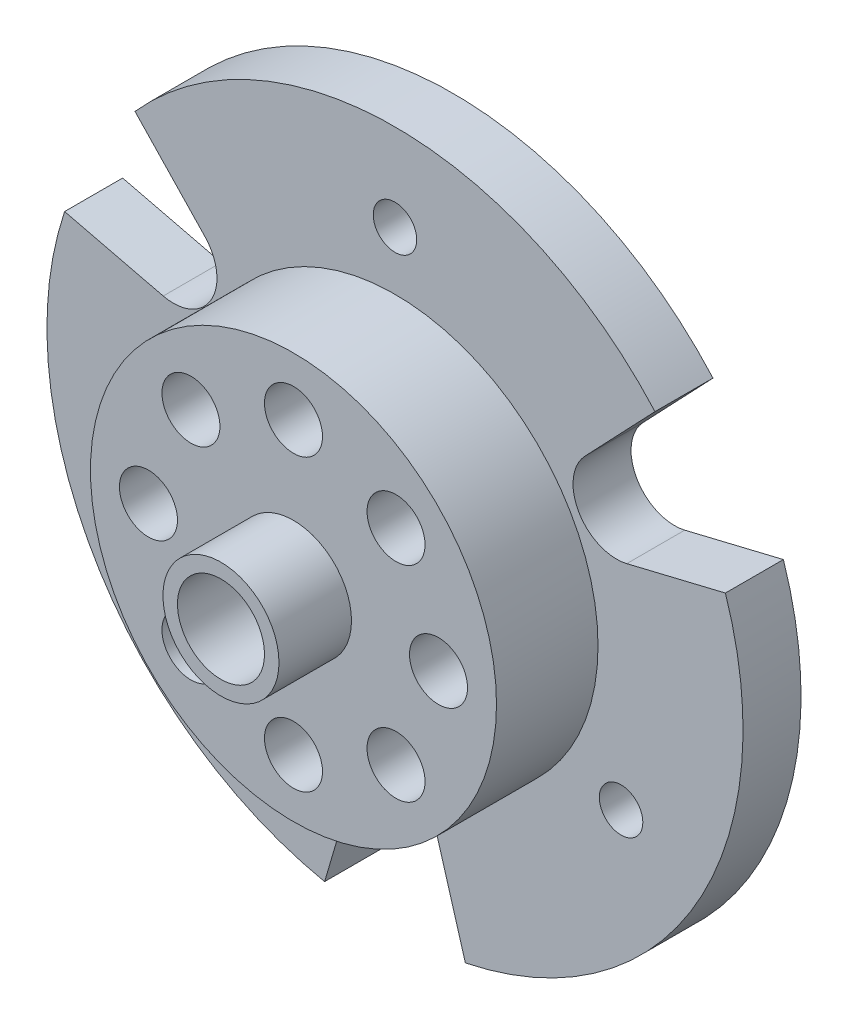
ISO-10303-21;
HEADER;
FILE_DESCRIPTION(('STEP AP214'),'2;1');
FILE_NAME('part.step','',(''),(''),'','','');
FILE_SCHEMA(('AUTOMOTIVE_DESIGN { 1 0 10303 214 1 1 1 1 }'));
ENDSEC;
DATA;
#1=APPLICATION_CONTEXT('core data for automotive mechanical design processes');
#2=APPLICATION_PROTOCOL_DEFINITION('international standard','automotive_design',2000,#1);
#3=PRODUCT_CONTEXT('',#1,'mechanical');
#4=PRODUCT('Part','Part','',(#3));
#5=PRODUCT_RELATED_PRODUCT_CATEGORY('part','',(#4));
#6=PRODUCT_DEFINITION_FORMATION('','',#4);
#7=PRODUCT_DEFINITION_CONTEXT('part definition',#1,'design');
#8=PRODUCT_DEFINITION('design','',#6,#7);
#9=PRODUCT_DEFINITION_SHAPE('','',#8);
#10=(LENGTH_UNIT() NAMED_UNIT(*) SI_UNIT(.MILLI.,.METRE.));
#11=(NAMED_UNIT(*) PLANE_ANGLE_UNIT() SI_UNIT($,.RADIAN.));
#12=(NAMED_UNIT(*) SI_UNIT($,.STERADIAN.) SOLID_ANGLE_UNIT());
#13=UNCERTAINTY_MEASURE_WITH_UNIT(LENGTH_MEASURE(1.E-05),#10,'distance_accuracy_value','');
#14=(GEOMETRIC_REPRESENTATION_CONTEXT(3) GLOBAL_UNCERTAINTY_ASSIGNED_CONTEXT((#13)) GLOBAL_UNIT_ASSIGNED_CONTEXT((#10,
#11,#12)) REPRESENTATION_CONTEXT('',''));
#15=CARTESIAN_POINT('',(0.,0.,0.));
#16=DIRECTION('',(0.,0.,1.));
#17=DIRECTION('',(1.,0.,0.));
#18=AXIS2_PLACEMENT_3D('',#15,#16,#17);
#19=CARTESIAN_POINT('',(0.,0.,4.));
#20=DIRECTION('',(0.,0.,-1.));
#21=DIRECTION('',(-1.,0.,0.));
#22=AXIS2_PLACEMENT_3D('',#19,#20,#21);
#23=CYLINDRICAL_SURFACE('',#22,24.);
#24=DIRECTION('',(0.,0.,1.));
#25=VECTOR('',#24,1.);
#26=CARTESIAN_POINT('',(-17.9280987104658,15.9556659725564,-26.));
#27=LINE('',#26,#25);
#28=CARTESIAN_POINT('',(-17.9280987104658,15.9556659725564,0.));
#29=VERTEX_POINT('',#28);
#30=CARTESIAN_POINT('',(-17.9280987104658,15.9556659725564,4.));
#31=VERTEX_POINT('',#30);
#32=EDGE_CURVE('E172',#29,#31,#27,.T.);
#33=ORIENTED_EDGE('',*,*,#32,.T.);
#34=CARTESIAN_POINT('',(0.,0.,4.));
#35=DIRECTION('',(0.,0.,1.));
#36=DIRECTION('',(1.,0.,0.));
#37=AXIS2_PLACEMENT_3D('',#34,#35,#36);
#38=CIRCLE('',#37,24.);
#39=CARTESIAN_POINT('',(17.928098710466,15.9556659725562,4.));
#40=VERTEX_POINT('',#39);
#41=EDGE_CURVE('E286',#40,#31,#38,.T.);
#42=ORIENTED_EDGE('',*,*,#41,.F.);
#43=DIRECTION('',(0.,0.,1.));
#44=VECTOR('',#43,1.);
#45=CARTESIAN_POINT('',(17.928098710466,15.9556659725562,-26.));
#46=LINE('',#45,#44);
#47=CARTESIAN_POINT('',(17.928098710466,15.9556659725562,0.));
#48=VERTEX_POINT('',#47);
#49=EDGE_CURVE('E162',#48,#40,#46,.T.);
#50=ORIENTED_EDGE('',*,*,#49,.F.);
#51=CARTESIAN_POINT('',(0.,0.,0.));
#52=DIRECTION('',(0.,0.,1.));
#53=DIRECTION('',(1.,0.,0.));
#54=AXIS2_PLACEMENT_3D('',#51,#52,#53);
#55=CIRCLE('',#54,24.);
#56=EDGE_CURVE('E291',#48,#29,#55,.T.);
#57=ORIENTED_EDGE('',*,*,#56,.T.);
#58=EDGE_LOOP('',(#33,#42,#50,#57));
#59=FACE_BOUND('',#58,.T.);
#60=ADVANCED_FACE('F60',(#59),#23,.T.);
#61=DIRECTION('',(0.,0.,1.));
#62=VECTOR('',#61,1.);
#63=CARTESIAN_POINT('',(22.7820614217657,7.5483559385401,-26.));
#64=LINE('',#63,#62);
#65=CARTESIAN_POINT('',(22.7820614217657,7.5483559385401,0.));
#66=VERTEX_POINT('',#65);
#67=CARTESIAN_POINT('',(22.7820614217657,7.5483559385401,4.));
#68=VERTEX_POINT('',#67);
#69=EDGE_CURVE('E187',#66,#68,#64,.T.);
#70=ORIENTED_EDGE('',*,*,#69,.T.);
#71=CARTESIAN_POINT('',(4.85396271129979,-23.5040219110966,4.));
#72=VERTEX_POINT('',#71);
#73=EDGE_CURVE('E289',#72,#68,#38,.T.);
#74=ORIENTED_EDGE('',*,*,#73,.F.);
#75=DIRECTION('',(0.,0.,1.));
#76=VECTOR('',#75,1.);
#77=CARTESIAN_POINT('',(4.85396271129979,-23.5040219110966,-26.));
#78=LINE('',#77,#76);
#79=CARTESIAN_POINT('',(4.85396271129979,-23.5040219110966,0.));
#80=VERTEX_POINT('',#79);
#81=EDGE_CURVE('E182',#80,#72,#78,.T.);
#82=ORIENTED_EDGE('',*,*,#81,.F.);
#83=EDGE_CURVE('E284',#80,#66,#55,.T.);
#84=ORIENTED_EDGE('',*,*,#83,.T.);
#85=EDGE_LOOP('',(#70,#74,#82,#84));
#86=FACE_BOUND('',#85,.T.);
#87=ADVANCED_FACE('F347',(#86),#23,.T.);
#88=CARTESIAN_POINT('',(-22.7820614217656,7.54835593854042,4.));
#89=VERTEX_POINT('',#88);
#90=CARTESIAN_POINT('',(-4.85396271129979,-23.5040219110967,4.));
#91=VERTEX_POINT('',#90);
#92=EDGE_CURVE('E295',#89,#91,#38,.T.);
#93=ORIENTED_EDGE('',*,*,#92,.F.);
#94=DIRECTION('',(0.,0.,1.));
#95=VECTOR('',#94,1.);
#96=CARTESIAN_POINT('',(-22.7820614217656,7.54835593854042,-26.));
#97=LINE('',#96,#95);
#98=CARTESIAN_POINT('',(-22.7820614217656,7.54835593854042,0.));
#99=VERTEX_POINT('',#98);
#100=EDGE_CURVE('E157',#99,#89,#97,.T.);
#101=ORIENTED_EDGE('',*,*,#100,.F.);
#102=CARTESIAN_POINT('',(-4.85396271129979,-23.5040219110967,0.));
#103=VERTEX_POINT('',#102);
#104=EDGE_CURVE('E298',#99,#103,#55,.T.);
#105=ORIENTED_EDGE('',*,*,#104,.T.);
#106=DIRECTION('',(0.,0.,1.));
#107=VECTOR('',#106,1.);
#108=CARTESIAN_POINT('',(-4.85396271129979,-23.5040219110967,-26.));
#109=LINE('',#108,#107);
#110=EDGE_CURVE('E204',#103,#91,#109,.T.);
#111=ORIENTED_EDGE('',*,*,#110,.T.);
#112=EDGE_LOOP('',(#93,#101,#105,#111));
#113=FACE_BOUND('',#112,.T.);
#114=ADVANCED_FACE('F56',(#113),#23,.T.);
#115=CARTESIAN_POINT('',(0.,0.,4.));
#116=DIRECTION('',(0.,0.,1.));
#117=DIRECTION('',(1.,0.,0.));
#118=AXIS2_PLACEMENT_3D('',#115,#116,#117);
#119=PLANE('',#118);
#120=DIRECTION('',(0.97198847965738,-0.235028499151349,0.));
#121=VECTOR('',#120,1.);
#122=CARTESIAN_POINT('',(0.465939606669434,1.92694899356498,4.));
#123=LINE('',#122,#121);
#124=CARTESIAN_POINT('',(-15.9817736202115,5.90403456102793,4.));
#125=VERTEX_POINT('',#124);
#126=EDGE_CURVE('E156',#89,#125,#123,.T.);
#127=ORIENTED_EDGE('',*,*,#126,.F.);
#128=ORIENTED_EDGE('',*,*,#92,.T.);
#129=DIRECTION('',(0.282453588950297,0.959280965144778,0.));
#130=VECTOR('',#129,1.);
#131=CARTESIAN_POINT('',(1.90175658355885,-0.559958960777444,4.));
#132=LINE('',#131,#130);
#133=CARTESIAN_POINT('',(-2.87784289543433,-16.7926392331491,4.));
#134=VERTEX_POINT('',#133);
#135=EDGE_CURVE('E200',#91,#134,#132,.T.);
#136=ORIENTED_EDGE('',*,*,#135,.T.);
#137=CARTESIAN_POINT('',(0.,-17.64,4.));
#138=DIRECTION('',(0.,0.,1.));
#139=DIRECTION('',(1.,0.,0.));
#140=AXIS2_PLACEMENT_3D('',#137,#138,#139);
#141=CIRCLE('',#140,3.);
#142=CARTESIAN_POINT('',(2.87784289543436,-16.7926392331492,4.));
#143=VERTEX_POINT('',#142);
#144=EDGE_CURVE('E198',#143,#134,#141,.T.);
#145=ORIENTED_EDGE('',*,*,#144,.F.);
#146=DIRECTION('',(-0.282453588950297,0.959280965144778,0.));
#147=VECTOR('',#146,1.);
#148=CARTESIAN_POINT('',(-1.90175658355885,-0.559958960777445,4.));
#149=LINE('',#148,#147);
#150=EDGE_CURVE('E191',#72,#143,#149,.T.);
#151=ORIENTED_EDGE('',*,*,#150,.F.);
#152=ORIENTED_EDGE('',*,*,#73,.T.);
#153=DIRECTION('',(-0.971988479657383,-0.235028499151335,0.));
#154=VECTOR('',#153,1.);
#155=CARTESIAN_POINT('',(-0.465939606669407,1.92694899356499,4.));
#156=LINE('',#155,#154);
#157=CARTESIAN_POINT('',(15.9817736202116,5.90403456102771,4.));
#158=VERTEX_POINT('',#157);
#159=EDGE_CURVE('E181',#68,#158,#156,.T.);
#160=ORIENTED_EDGE('',*,*,#159,.T.);
#161=CARTESIAN_POINT('',(15.2766881227576,8.81999999999986,4.));
#162=DIRECTION('',(0.,0.,1.));
#163=DIRECTION('',(1.,0.,0.));
#164=AXIS2_PLACEMENT_3D('',#161,#162,#163);
#165=CIRCLE('',#164,3.);
#166=CARTESIAN_POINT('',(13.1039307247773,10.8886046721211,4.));
#167=VERTEX_POINT('',#166);
#168=EDGE_CURVE('E177',#167,#158,#165,.T.);
#169=ORIENTED_EDGE('',*,*,#168,.F.);
#170=DIRECTION('',(-0.689534890707091,-0.724252465993427,0.));
#171=VECTOR('',#170,1.);
#172=CARTESIAN_POINT('',(1.43581697688941,-1.36699003278756,4.));
#173=LINE('',#172,#171);
#174=EDGE_CURVE('E180',#40,#167,#173,.T.);
#175=ORIENTED_EDGE('',*,*,#174,.F.);
#176=ORIENTED_EDGE('',*,*,#41,.T.);
#177=DIRECTION('',(0.689534890707081,-0.724252465993437,0.));
#178=VECTOR('',#177,1.);
#179=CARTESIAN_POINT('',(-1.43581697688943,-1.36699003278754,4.));
#180=LINE('',#179,#178);
#181=CARTESIAN_POINT('',(-13.1039307247772,10.8886046721213,4.));
#182=VERTEX_POINT('',#181);
#183=EDGE_CURVE('E153',#31,#182,#180,.T.);
#184=ORIENTED_EDGE('',*,*,#183,.T.);
#185=CARTESIAN_POINT('',(-15.2766881227575,8.82,4.));
#186=DIRECTION('',(0.,0.,1.));
#187=DIRECTION('',(1.,0.,0.));
#188=AXIS2_PLACEMENT_3D('',#185,#186,#187);
#189=CIRCLE('',#188,3.);
#190=EDGE_CURVE('E146',#125,#182,#189,.T.);
#191=ORIENTED_EDGE('',*,*,#190,.F.);
#192=EDGE_LOOP('',(#127,#128,#136,#145,#151,#152,#160,#169,#175,#176,#184,#191));
#193=FACE_BOUND('',#192,.T.);
#194=CARTESIAN_POINT('',(-15.5884572681187,-9.00000000000067,4.));
#195=DIRECTION('',(0.,0.,1.));
#196=DIRECTION('',(1.,0.,0.));
#197=AXIS2_PLACEMENT_3D('',#194,#195,#196);
#198=CIRCLE('',#197,1.50000000000146);
#199=CARTESIAN_POINT('',(-14.0884572681173,-9.00000000000067,4.));
#200=VERTEX_POINT('',#199);
#201=EDGE_CURVE('E269',#200,#200,#198,.T.);
#202=ORIENTED_EDGE('',*,*,#201,.F.);
#203=EDGE_LOOP('',(#202));
#204=FACE_BOUND('',#203,.T.);
#205=CARTESIAN_POINT('',(15.588457268121,-8.99999999999934,4.));
#206=DIRECTION('',(0.,0.,1.));
#207=DIRECTION('',(1.,0.,0.));
#208=AXIS2_PLACEMENT_3D('',#205,#206,#207);
#209=CIRCLE('',#208,1.50000000000099);
#210=CARTESIAN_POINT('',(17.088457268122,-8.99999999999934,4.));
#211=VERTEX_POINT('',#210);
#212=EDGE_CURVE('E273',#211,#211,#209,.T.);
#213=ORIENTED_EDGE('',*,*,#212,.F.);
#214=EDGE_LOOP('',(#213));
#215=FACE_BOUND('',#214,.T.);
#216=CARTESIAN_POINT('',(0.,18.,4.));
#217=DIRECTION('',(0.,0.,1.));
#218=DIRECTION('',(1.,0.,0.));
#219=AXIS2_PLACEMENT_3D('',#216,#217,#218);
#220=CIRCLE('',#219,1.5);
#221=CARTESIAN_POINT('',(1.5,18.,4.));
#222=VERTEX_POINT('',#221);
#223=EDGE_CURVE('E270',#222,#222,#220,.T.);
#224=ORIENTED_EDGE('',*,*,#223,.F.);
#225=EDGE_LOOP('',(#224));
#226=FACE_BOUND('',#225,.T.);
#227=CARTESIAN_POINT('',(0.,0.,4.));
#228=DIRECTION('',(0.,0.,1.));
#229=DIRECTION('',(1.,0.,0.));
#230=AXIS2_PLACEMENT_3D('',#227,#228,#229);
#231=CIRCLE('',#230,14.);
#232=CARTESIAN_POINT('',(14.,0.,4.));
#233=VERTEX_POINT('',#232);
#234=EDGE_CURVE('E285',#233,#233,#231,.T.);
#235=ORIENTED_EDGE('',*,*,#234,.F.);
#236=EDGE_LOOP('',(#235));
#237=FACE_BOUND('',#236,.T.);
#238=ADVANCED_FACE('F164',(#193,#204,#215,#226,#237),#119,.T.);
#239=CARTESIAN_POINT('',(0.,0.,0.));
#240=DIRECTION('',(0.,0.,1.));
#241=DIRECTION('',(1.,0.,0.));
#242=AXIS2_PLACEMENT_3D('',#239,#240,#241);
#243=PLANE('',#242);
#244=CARTESIAN_POINT('',(0.,0.,0.));
#245=DIRECTION('',(0.,0.,1.));
#246=DIRECTION('',(1.,0.,0.));
#247=AXIS2_PLACEMENT_3D('',#244,#245,#246);
#248=CIRCLE('',#247,3.);
#249=CARTESIAN_POINT('',(3.,0.,0.));
#250=VERTEX_POINT('',#249);
#251=EDGE_CURVE('E215',#250,#250,#248,.T.);
#252=ORIENTED_EDGE('',*,*,#251,.T.);
#253=EDGE_LOOP('',(#252));
#254=FACE_BOUND('',#253,.T.);
#255=CARTESIAN_POINT('',(-15.5884572681187,-9.00000000000067,0.));
#256=DIRECTION('',(0.,0.,1.));
#257=DIRECTION('',(1.,0.,0.));
#258=AXIS2_PLACEMENT_3D('',#255,#256,#257);
#259=CIRCLE('',#258,1.50000000000146);
#260=CARTESIAN_POINT('',(-14.0884572681173,-9.00000000000067,0.));
#261=VERTEX_POINT('',#260);
#262=EDGE_CURVE('E282',#261,#261,#259,.T.);
#263=ORIENTED_EDGE('',*,*,#262,.T.);
#264=EDGE_LOOP('',(#263));
#265=FACE_BOUND('',#264,.T.);
#266=CARTESIAN_POINT('',(15.588457268121,-8.99999999999934,0.));
#267=DIRECTION('',(0.,0.,1.));
#268=DIRECTION('',(1.,0.,0.));
#269=AXIS2_PLACEMENT_3D('',#266,#267,#268);
#270=CIRCLE('',#269,1.50000000000099);
#271=CARTESIAN_POINT('',(17.088457268122,-8.99999999999934,0.));
#272=VERTEX_POINT('',#271);
#273=EDGE_CURVE('E300',#272,#272,#270,.T.);
#274=ORIENTED_EDGE('',*,*,#273,.T.);
#275=EDGE_LOOP('',(#274));
#276=FACE_BOUND('',#275,.T.);
#277=CARTESIAN_POINT('',(0.,18.,0.));
#278=DIRECTION('',(0.,0.,1.));
#279=DIRECTION('',(1.,0.,0.));
#280=AXIS2_PLACEMENT_3D('',#277,#278,#279);
#281=CIRCLE('',#280,1.5);
#282=CARTESIAN_POINT('',(1.5,18.,0.));
#283=VERTEX_POINT('',#282);
#284=EDGE_CURVE('E272',#283,#283,#281,.T.);
#285=ORIENTED_EDGE('',*,*,#284,.T.);
#286=EDGE_LOOP('',(#285));
#287=FACE_BOUND('',#286,.T.);
#288=ORIENTED_EDGE('',*,*,#104,.F.);
#289=DIRECTION('',(0.97198847965738,-0.235028499151349,0.));
#290=VECTOR('',#289,1.);
#291=CARTESIAN_POINT('',(0.465939606669434,1.92694899356498,0.));
#292=LINE('',#291,#290);
#293=CARTESIAN_POINT('',(-15.9817736202115,5.90403456102793,0.));
#294=VERTEX_POINT('',#293);
#295=EDGE_CURVE('E12',#99,#294,#292,.T.);
#296=ORIENTED_EDGE('',*,*,#295,.T.);
#297=CARTESIAN_POINT('',(-15.2766881227575,8.82,0.));
#298=DIRECTION('',(0.,0.,1.));
#299=DIRECTION('',(1.,0.,0.));
#300=AXIS2_PLACEMENT_3D('',#297,#298,#299);
#301=CIRCLE('',#300,3.);
#302=CARTESIAN_POINT('',(-13.1039307247772,10.8886046721213,0.));
#303=VERTEX_POINT('',#302);
#304=EDGE_CURVE('E151',#294,#303,#301,.T.);
#305=ORIENTED_EDGE('',*,*,#304,.T.);
#306=DIRECTION('',(0.689534890707081,-0.724252465993437,0.));
#307=VECTOR('',#306,1.);
#308=CARTESIAN_POINT('',(-1.43581697688943,-1.36699003278754,0.));
#309=LINE('',#308,#307);
#310=EDGE_CURVE('E61',#29,#303,#309,.T.);
#311=ORIENTED_EDGE('',*,*,#310,.F.);
#312=ORIENTED_EDGE('',*,*,#56,.F.);
#313=DIRECTION('',(-0.689534890707091,-0.724252465993427,0.));
#314=VECTOR('',#313,1.);
#315=CARTESIAN_POINT('',(1.43581697688941,-1.36699003278756,0.));
#316=LINE('',#315,#314);
#317=CARTESIAN_POINT('',(13.1039307247773,10.8886046721211,0.));
#318=VERTEX_POINT('',#317);
#319=EDGE_CURVE('E320',#48,#318,#316,.T.);
#320=ORIENTED_EDGE('',*,*,#319,.T.);
#321=CARTESIAN_POINT('',(15.2766881227576,8.81999999999986,0.));
#322=DIRECTION('',(0.,0.,1.));
#323=DIRECTION('',(1.,0.,0.));
#324=AXIS2_PLACEMENT_3D('',#321,#322,#323);
#325=CIRCLE('',#324,3.);
#326=CARTESIAN_POINT('',(15.9817736202116,5.9040345610277,0.));
#327=VERTEX_POINT('',#326);
#328=EDGE_CURVE('E315',#318,#327,#325,.T.);
#329=ORIENTED_EDGE('',*,*,#328,.T.);
#330=DIRECTION('',(-0.971988479657383,-0.235028499151335,0.));
#331=VECTOR('',#330,1.);
#332=CARTESIAN_POINT('',(-0.465939606669407,1.92694899356499,0.));
#333=LINE('',#332,#331);
#334=EDGE_CURVE('E312',#66,#327,#333,.T.);
#335=ORIENTED_EDGE('',*,*,#334,.F.);
#336=ORIENTED_EDGE('',*,*,#83,.F.);
#337=DIRECTION('',(-0.282453588950297,0.959280965144778,0.));
#338=VECTOR('',#337,1.);
#339=CARTESIAN_POINT('',(-1.90175658355885,-0.559958960777445,0.));
#340=LINE('',#339,#338);
#341=CARTESIAN_POINT('',(2.87784289543436,-16.7926392331492,0.));
#342=VERTEX_POINT('',#341);
#343=EDGE_CURVE('E310',#80,#342,#340,.T.);
#344=ORIENTED_EDGE('',*,*,#343,.T.);
#345=CARTESIAN_POINT('',(0.,-17.64,0.));
#346=DIRECTION('',(0.,0.,1.));
#347=DIRECTION('',(1.,0.,0.));
#348=AXIS2_PLACEMENT_3D('',#345,#346,#347);
#349=CIRCLE('',#348,3.);
#350=CARTESIAN_POINT('',(-2.87784289543433,-16.7926392331491,0.));
#351=VERTEX_POINT('',#350);
#352=EDGE_CURVE('E290',#342,#351,#349,.T.);
#353=ORIENTED_EDGE('',*,*,#352,.T.);
#354=DIRECTION('',(0.282453588950297,0.959280965144778,0.));
#355=VECTOR('',#354,1.);
#356=CARTESIAN_POINT('',(1.90175658355885,-0.559958960777444,0.));
#357=LINE('',#356,#355);
#358=EDGE_CURVE('E308',#103,#351,#357,.T.);
#359=ORIENTED_EDGE('',*,*,#358,.F.);
#360=EDGE_LOOP('',(#288,#296,#305,#311,#312,#320,#329,#335,#336,#344,#353,#359));
#361=FACE_BOUND('',#360,.T.);
#362=ADVANCED_FACE('F330',(#254,#265,#276,#287,#361),#243,.F.);
#363=CARTESIAN_POINT('',(0.,0.,11.));
#364=DIRECTION('',(0.,0.,-1.));
#365=DIRECTION('',(-1.,0.,0.));
#366=AXIS2_PLACEMENT_3D('',#363,#364,#365);
#367=CYLINDRICAL_SURFACE('',#366,14.);
#368=CARTESIAN_POINT('',(0.,0.,11.));
#369=DIRECTION('',(0.,0.,1.));
#370=DIRECTION('',(1.,0.,0.));
#371=AXIS2_PLACEMENT_3D('',#368,#369,#370);
#372=CIRCLE('',#371,14.);
#373=CARTESIAN_POINT('',(14.,0.,11.));
#374=VERTEX_POINT('',#373);
#375=EDGE_CURVE('E276',#374,#374,#372,.T.);
#376=ORIENTED_EDGE('',*,*,#375,.F.);
#377=EDGE_LOOP('',(#376));
#378=FACE_BOUND('',#377,.T.);
#379=ORIENTED_EDGE('',*,*,#234,.T.);
#380=EDGE_LOOP('',(#379));
#381=FACE_BOUND('',#380,.T.);
#382=ADVANCED_FACE('F379',(#378,#381),#367,.T.);
#383=CARTESIAN_POINT('',(0.,0.,11.));
#384=DIRECTION('',(0.,0.,1.));
#385=DIRECTION('',(1.,0.,0.));
#386=AXIS2_PLACEMENT_3D('',#383,#384,#385);
#387=PLANE('',#386);
#388=CARTESIAN_POINT('',(0.,0.,11.));
#389=DIRECTION('',(0.,0.,1.));
#390=DIRECTION('',(1.,0.,0.));
#391=AXIS2_PLACEMENT_3D('',#388,#389,#390);
#392=CIRCLE('',#391,4.);
#393=CARTESIAN_POINT('',(4.,0.,11.));
#394=VERTEX_POINT('',#393);
#395=EDGE_CURVE('E214',#394,#394,#392,.T.);
#396=ORIENTED_EDGE('',*,*,#395,.F.);
#397=EDGE_LOOP('',(#396));
#398=FACE_BOUND('',#397,.T.);
#399=CARTESIAN_POINT('',(-7.07106781186535,7.07106781186517,11.));
#400=DIRECTION('',(0.,0.,1.));
#401=DIRECTION('',(1.,0.,0.));
#402=AXIS2_PLACEMENT_3D('',#399,#400,#401);
#403=CIRCLE('',#402,2.00000000000032);
#404=CARTESIAN_POINT('',(-5.07106781186503,7.07106781186517,11.));
#405=VERTEX_POINT('',#404);
#406=EDGE_CURVE('E238',#405,#405,#403,.T.);
#407=ORIENTED_EDGE('',*,*,#406,.F.);
#408=EDGE_LOOP('',(#407));
#409=FACE_BOUND('',#408,.T.);
#410=CARTESIAN_POINT('',(-9.99999999999958,-4.25713318056486E-13,11.));
#411=DIRECTION('',(0.,0.,1.));
#412=DIRECTION('',(1.,0.,0.));
#413=AXIS2_PLACEMENT_3D('',#410,#411,#412);
#414=CIRCLE('',#413,2.00000000000063);
#415=CARTESIAN_POINT('',(-7.99999999999895,-4.25713318056486E-13,11.));
#416=VERTEX_POINT('',#415);
#417=EDGE_CURVE('E250',#416,#416,#414,.T.);
#418=ORIENTED_EDGE('',*,*,#417,.F.);
#419=EDGE_LOOP('',(#418));
#420=FACE_BOUND('',#419,.T.);
#421=CARTESIAN_POINT('',(7.0710678118662,-7.07106781186517,11.));
#422=DIRECTION('',(0.,0.,1.));
#423=DIRECTION('',(1.,0.,0.));
#424=AXIS2_PLACEMENT_3D('',#421,#422,#423);
#425=CIRCLE('',#424,2.00000000000066);
#426=CARTESIAN_POINT('',(9.07106781186686,-7.07106781186517,11.));
#427=VERTEX_POINT('',#426);
#428=EDGE_CURVE('E251',#427,#427,#425,.T.);
#429=ORIENTED_EDGE('',*,*,#428,.F.);
#430=EDGE_LOOP('',(#429));
#431=FACE_BOUND('',#430,.T.);
#432=CARTESIAN_POINT('',(8.48977342514678E-13,-10.,11.));
#433=DIRECTION('',(0.,0.,1.));
#434=DIRECTION('',(1.,0.,0.));
#435=AXIS2_PLACEMENT_3D('',#432,#433,#434);
#436=CIRCLE('',#435,2.00000000000088);
#437=CARTESIAN_POINT('',(2.00000000000173,-10.,11.));
#438=VERTEX_POINT('',#437);
#439=EDGE_CURVE('E259',#438,#438,#436,.T.);
#440=ORIENTED_EDGE('',*,*,#439,.F.);
#441=EDGE_LOOP('',(#440));
#442=FACE_BOUND('',#441,.T.);
#443=CARTESIAN_POINT('',(0.,10.,11.));
#444=DIRECTION('',(0.,0.,1.));
#445=DIRECTION('',(1.,0.,0.));
#446=AXIS2_PLACEMENT_3D('',#443,#444,#445);
#447=CIRCLE('',#446,2.);
#448=CARTESIAN_POINT('',(2.,10.,11.));
#449=VERTEX_POINT('',#448);
#450=EDGE_CURVE('E225',#449,#449,#447,.T.);
#451=ORIENTED_EDGE('',*,*,#450,.F.);
#452=EDGE_LOOP('',(#451));
#453=FACE_BOUND('',#452,.T.);
#454=CARTESIAN_POINT('',(7.0710678118656,7.07106781186578,11.));
#455=DIRECTION('',(0.,0.,1.));
#456=DIRECTION('',(1.,0.,0.));
#457=AXIS2_PLACEMENT_3D('',#454,#455,#456);
#458=CIRCLE('',#457,2.00000000000005);
#459=CARTESIAN_POINT('',(9.07106781186565,7.07106781186578,11.));
#460=VERTEX_POINT('',#459);
#461=EDGE_CURVE('E232',#460,#460,#458,.T.);
#462=ORIENTED_EDGE('',*,*,#461,.F.);
#463=EDGE_LOOP('',(#462));
#464=FACE_BOUND('',#463,.T.);
#465=CARTESIAN_POINT('',(-7.07106781186475,-7.07106781186578,11.));
#466=DIRECTION('',(0.,0.,1.));
#467=DIRECTION('',(1.,0.,0.));
#468=AXIS2_PLACEMENT_3D('',#465,#466,#467);
#469=CIRCLE('',#468,2.00000000000086);
#470=CARTESIAN_POINT('',(-5.07106781186389,-7.07106781186578,11.));
#471=VERTEX_POINT('',#470);
#472=EDGE_CURVE('E227',#471,#471,#469,.T.);
#473=ORIENTED_EDGE('',*,*,#472,.F.);
#474=EDGE_LOOP('',(#473));
#475=FACE_BOUND('',#474,.T.);
#476=CARTESIAN_POINT('',(10.0000000000004,4.24488671257339E-13,11.));
#477=DIRECTION('',(0.,0.,1.));
#478=DIRECTION('',(1.,0.,0.));
#479=AXIS2_PLACEMENT_3D('',#476,#477,#478);
#480=CIRCLE('',#479,2.00000000000031);
#481=CARTESIAN_POINT('',(12.0000000000007,4.24488671257339E-13,11.));
#482=VERTEX_POINT('',#481);
#483=EDGE_CURVE('E242',#482,#482,#480,.T.);
#484=ORIENTED_EDGE('',*,*,#483,.F.);
#485=EDGE_LOOP('',(#484));
#486=FACE_BOUND('',#485,.T.);
#487=ORIENTED_EDGE('',*,*,#375,.T.);
#488=EDGE_LOOP('',(#487));
#489=FACE_BOUND('',#488,.T.);
#490=ADVANCED_FACE('F384',(#398,#409,#420,#431,#442,#453,#464,#475,#486,#489),#387,.T.);
#491=CARTESIAN_POINT('',(0.,18.,-6.));
#492=DIRECTION('',(0.,0.,1.));
#493=DIRECTION('',(1.,0.,0.));
#494=AXIS2_PLACEMENT_3D('',#491,#492,#493);
#495=CYLINDRICAL_SURFACE('',#494,1.5);
#496=ORIENTED_EDGE('',*,*,#223,.T.);
#497=EDGE_LOOP('',(#496));
#498=FACE_BOUND('',#497,.T.);
#499=ORIENTED_EDGE('',*,*,#284,.F.);
#500=EDGE_LOOP('',(#499));
#501=FACE_BOUND('',#500,.T.);
#502=ADVANCED_FACE('F386',(#498,#501),#495,.F.);
#503=CARTESIAN_POINT('',(15.588457268121,-8.99999999999934,-6.));
#504=DIRECTION('',(0.,0.,1.));
#505=DIRECTION('',(1.,0.,0.));
#506=AXIS2_PLACEMENT_3D('',#503,#504,#505);
#507=CYLINDRICAL_SURFACE('',#506,1.50000000000099);
#508=ORIENTED_EDGE('',*,*,#212,.T.);
#509=EDGE_LOOP('',(#508));
#510=FACE_BOUND('',#509,.T.);
#511=ORIENTED_EDGE('',*,*,#273,.F.);
#512=EDGE_LOOP('',(#511));
#513=FACE_BOUND('',#512,.T.);
#514=ADVANCED_FACE('F392',(#510,#513),#507,.F.);
#515=CARTESIAN_POINT('',(-15.5884572681187,-9.00000000000067,-6.));
#516=DIRECTION('',(0.,0.,1.));
#517=DIRECTION('',(1.,0.,0.));
#518=AXIS2_PLACEMENT_3D('',#515,#516,#517);
#519=CYLINDRICAL_SURFACE('',#518,1.50000000000146);
#520=ORIENTED_EDGE('',*,*,#201,.T.);
#521=EDGE_LOOP('',(#520));
#522=FACE_BOUND('',#521,.T.);
#523=ORIENTED_EDGE('',*,*,#262,.F.);
#524=EDGE_LOOP('',(#523));
#525=FACE_BOUND('',#524,.T.);
#526=ADVANCED_FACE('F400',(#522,#525),#519,.F.);
#527=CARTESIAN_POINT('',(10.0000000000004,4.24488671257339E-13,0.999999999999999));
#528=DIRECTION('',(0.,0.,1.));
#529=DIRECTION('',(1.,0.,0.));
#530=AXIS2_PLACEMENT_3D('',#527,#528,#529);
#531=CYLINDRICAL_SURFACE('',#530,2.00000000000031);
#532=ORIENTED_EDGE('',*,*,#483,.T.);
#533=EDGE_LOOP('',(#532));
#534=FACE_BOUND('',#533,.T.);
#535=CARTESIAN_POINT('',(10.0000000000004,4.24488671257339E-13,0.999999999999999));
#536=DIRECTION('',(0.,0.,1.));
#537=DIRECTION('',(1.,0.,0.));
#538=AXIS2_PLACEMENT_3D('',#535,#536,#537);
#539=CIRCLE('',#538,2.00000000000031);
#540=CARTESIAN_POINT('',(12.0000000000007,4.24488671257339E-13,0.999999999999999));
#541=VERTEX_POINT('',#540);
#542=EDGE_CURVE('E262',#541,#541,#539,.T.);
#543=ORIENTED_EDGE('',*,*,#542,.F.);
#544=EDGE_LOOP('',(#543));
#545=FACE_BOUND('',#544,.T.);
#546=ADVANCED_FACE('F402',(#534,#545),#531,.F.);
#547=CARTESIAN_POINT('',(0.,0.,0.999999999999999));
#548=DIRECTION('',(0.,0.,1.));
#549=DIRECTION('',(1.,0.,0.));
#550=AXIS2_PLACEMENT_3D('',#547,#548,#549);
#551=PLANE('',#550);
#552=ORIENTED_EDGE('',*,*,#542,.T.);
#553=EDGE_LOOP('',(#552));
#554=FACE_BOUND('',#553,.T.);
#555=ADVANCED_FACE('F403',(#554),#551,.T.);
#556=CARTESIAN_POINT('',(-7.07106781186475,-7.07106781186578,0.999999999999999));
#557=DIRECTION('',(0.,0.,1.));
#558=DIRECTION('',(1.,0.,0.));
#559=AXIS2_PLACEMENT_3D('',#556,#557,#558);
#560=CYLINDRICAL_SURFACE('',#559,2.00000000000086);
#561=CARTESIAN_POINT('',(-7.07106781186475,-7.07106781186578,0.999999999999999));
#562=DIRECTION('',(0.,0.,1.));
#563=DIRECTION('',(1.,0.,0.));
#564=AXIS2_PLACEMENT_3D('',#561,#562,#563);
#565=CIRCLE('',#564,2.00000000000086);
#566=CARTESIAN_POINT('',(-5.07106781186389,-7.07106781186578,0.999999999999999));
#567=VERTEX_POINT('',#566);
#568=EDGE_CURVE('E235',#567,#567,#565,.T.);
#569=ORIENTED_EDGE('',*,*,#568,.F.);
#570=EDGE_LOOP('',(#569));
#571=FACE_BOUND('',#570,.T.);
#572=ORIENTED_EDGE('',*,*,#472,.T.);
#573=EDGE_LOOP('',(#572));
#574=FACE_BOUND('',#573,.T.);
#575=ADVANCED_FACE('F410',(#571,#574),#560,.F.);
#576=CARTESIAN_POINT('',(0.,0.,0.999999999999999));
#577=DIRECTION('',(0.,0.,1.));
#578=DIRECTION('',(1.,0.,0.));
#579=AXIS2_PLACEMENT_3D('',#576,#577,#578);
#580=PLANE('',#579);
#581=ORIENTED_EDGE('',*,*,#568,.T.);
#582=EDGE_LOOP('',(#581));
#583=FACE_BOUND('',#582,.T.);
#584=ADVANCED_FACE('F451',(#583),#580,.T.);
#585=CARTESIAN_POINT('',(7.0710678118656,7.07106781186578,0.999999999999999));
#586=DIRECTION('',(0.,0.,1.));
#587=DIRECTION('',(1.,0.,0.));
#588=AXIS2_PLACEMENT_3D('',#585,#586,#587);
#589=CYLINDRICAL_SURFACE('',#588,2.00000000000005);
#590=CARTESIAN_POINT('',(7.0710678118656,7.07106781186578,0.999999999999999));
#591=DIRECTION('',(0.,0.,1.));
#592=DIRECTION('',(1.,0.,0.));
#593=AXIS2_PLACEMENT_3D('',#590,#591,#592);
#594=CIRCLE('',#593,2.00000000000005);
#595=CARTESIAN_POINT('',(9.07106781186565,7.07106781186578,0.999999999999999));
#596=VERTEX_POINT('',#595);
#597=EDGE_CURVE('E223',#596,#596,#594,.T.);
#598=ORIENTED_EDGE('',*,*,#597,.F.);
#599=EDGE_LOOP('',(#598));
#600=FACE_BOUND('',#599,.T.);
#601=ORIENTED_EDGE('',*,*,#461,.T.);
#602=EDGE_LOOP('',(#601));
#603=FACE_BOUND('',#602,.T.);
#604=ADVANCED_FACE('F450',(#600,#603),#589,.F.);
#605=CARTESIAN_POINT('',(0.,0.,0.999999999999999));
#606=DIRECTION('',(0.,0.,1.));
#607=DIRECTION('',(1.,0.,0.));
#608=AXIS2_PLACEMENT_3D('',#605,#606,#607);
#609=PLANE('',#608);
#610=ORIENTED_EDGE('',*,*,#597,.T.);
#611=EDGE_LOOP('',(#610));
#612=FACE_BOUND('',#611,.T.);
#613=ADVANCED_FACE('F443',(#612),#609,.T.);
#614=CARTESIAN_POINT('',(0.,10.,0.999999999999999));
#615=DIRECTION('',(0.,0.,1.));
#616=DIRECTION('',(1.,0.,0.));
#617=AXIS2_PLACEMENT_3D('',#614,#615,#616);
#618=CYLINDRICAL_SURFACE('',#617,2.);
#619=ORIENTED_EDGE('',*,*,#450,.T.);
#620=EDGE_LOOP('',(#619));
#621=FACE_BOUND('',#620,.T.);
#622=CARTESIAN_POINT('',(0.,10.,0.999999999999999));
#623=DIRECTION('',(0.,0.,1.));
#624=DIRECTION('',(1.,0.,0.));
#625=AXIS2_PLACEMENT_3D('',#622,#623,#624);
#626=CIRCLE('',#625,2.);
#627=CARTESIAN_POINT('',(2.,10.,0.999999999999999));
#628=VERTEX_POINT('',#627);
#629=EDGE_CURVE('E218',#628,#628,#626,.T.);
#630=ORIENTED_EDGE('',*,*,#629,.F.);
#631=EDGE_LOOP('',(#630));
#632=FACE_BOUND('',#631,.T.);
#633=ADVANCED_FACE('F447',(#621,#632),#618,.F.);
#634=CARTESIAN_POINT('',(0.,0.,0.999999999999999));
#635=DIRECTION('',(0.,0.,1.));
#636=DIRECTION('',(1.,0.,0.));
#637=AXIS2_PLACEMENT_3D('',#634,#635,#636);
#638=PLANE('',#637);
#639=ORIENTED_EDGE('',*,*,#629,.T.);
#640=EDGE_LOOP('',(#639));
#641=FACE_BOUND('',#640,.T.);
#642=ADVANCED_FACE('F420',(#641),#638,.T.);
#643=CARTESIAN_POINT('',(8.48977342514678E-13,-10.,0.999999999999999));
#644=DIRECTION('',(0.,0.,1.));
#645=DIRECTION('',(1.,0.,0.));
#646=AXIS2_PLACEMENT_3D('',#643,#644,#645);
#647=CYLINDRICAL_SURFACE('',#646,2.00000000000088);
#648=CARTESIAN_POINT('',(8.48977342514678E-13,-10.,0.999999999999999));
#649=DIRECTION('',(0.,0.,1.));
#650=DIRECTION('',(1.,0.,0.));
#651=AXIS2_PLACEMENT_3D('',#648,#649,#650);
#652=CIRCLE('',#651,2.00000000000088);
#653=CARTESIAN_POINT('',(2.00000000000173,-10.,0.999999999999999));
#654=VERTEX_POINT('',#653);
#655=EDGE_CURVE('E233',#654,#654,#652,.T.);
#656=ORIENTED_EDGE('',*,*,#655,.F.);
#657=EDGE_LOOP('',(#656));
#658=FACE_BOUND('',#657,.T.);
#659=ORIENTED_EDGE('',*,*,#439,.T.);
#660=EDGE_LOOP('',(#659));
#661=FACE_BOUND('',#660,.T.);
#662=ADVANCED_FACE('F412',(#658,#661),#647,.F.);
#663=CARTESIAN_POINT('',(0.,0.,0.999999999999999));
#664=DIRECTION('',(0.,0.,1.));
#665=DIRECTION('',(1.,0.,0.));
#666=AXIS2_PLACEMENT_3D('',#663,#664,#665);
#667=PLANE('',#666);
#668=ORIENTED_EDGE('',*,*,#655,.T.);
#669=EDGE_LOOP('',(#668));
#670=FACE_BOUND('',#669,.T.);
#671=ADVANCED_FACE('F413',(#670),#667,.T.);
#672=CARTESIAN_POINT('',(7.0710678118662,-7.07106781186517,0.999999999999999));
#673=DIRECTION('',(0.,0.,1.));
#674=DIRECTION('',(1.,0.,0.));
#675=AXIS2_PLACEMENT_3D('',#672,#673,#674);
#676=CYLINDRICAL_SURFACE('',#675,2.00000000000066);
#677=CARTESIAN_POINT('',(7.0710678118662,-7.07106781186517,0.999999999999999));
#678=DIRECTION('',(0.,0.,1.));
#679=DIRECTION('',(1.,0.,0.));
#680=AXIS2_PLACEMENT_3D('',#677,#678,#679);
#681=CIRCLE('',#680,2.00000000000066);
#682=CARTESIAN_POINT('',(9.07106781186686,-7.07106781186517,0.999999999999999));
#683=VERTEX_POINT('',#682);
#684=EDGE_CURVE('E258',#683,#683,#681,.T.);
#685=ORIENTED_EDGE('',*,*,#684,.F.);
#686=EDGE_LOOP('',(#685));
#687=FACE_BOUND('',#686,.T.);
#688=ORIENTED_EDGE('',*,*,#428,.T.);
#689=EDGE_LOOP('',(#688));
#690=FACE_BOUND('',#689,.T.);
#691=ADVANCED_FACE('F414',(#687,#690),#676,.F.);
#692=CARTESIAN_POINT('',(0.,0.,0.999999999999999));
#693=DIRECTION('',(0.,0.,1.));
#694=DIRECTION('',(1.,0.,0.));
#695=AXIS2_PLACEMENT_3D('',#692,#693,#694);
#696=PLANE('',#695);
#697=ORIENTED_EDGE('',*,*,#684,.T.);
#698=EDGE_LOOP('',(#697));
#699=FACE_BOUND('',#698,.T.);
#700=ADVANCED_FACE('F423',(#699),#696,.T.);
#701=CARTESIAN_POINT('',(-9.99999999999958,-4.25713318056486E-13,0.999999999999999));
#702=DIRECTION('',(0.,0.,1.));
#703=DIRECTION('',(1.,0.,0.));
#704=AXIS2_PLACEMENT_3D('',#701,#702,#703);
#705=CYLINDRICAL_SURFACE('',#704,2.00000000000063);
#706=CARTESIAN_POINT('',(-9.99999999999958,-4.25713318056486E-13,0.999999999999999));
#707=DIRECTION('',(0.,0.,1.));
#708=DIRECTION('',(1.,0.,0.));
#709=AXIS2_PLACEMENT_3D('',#706,#707,#708);
#710=CIRCLE('',#709,2.00000000000063);
#711=CARTESIAN_POINT('',(-7.99999999999895,-4.25713318056486E-13,0.999999999999999));
#712=VERTEX_POINT('',#711);
#713=EDGE_CURVE('E247',#712,#712,#710,.T.);
#714=ORIENTED_EDGE('',*,*,#713,.F.);
#715=EDGE_LOOP('',(#714));
#716=FACE_BOUND('',#715,.T.);
#717=ORIENTED_EDGE('',*,*,#417,.T.);
#718=EDGE_LOOP('',(#717));
#719=FACE_BOUND('',#718,.T.);
#720=ADVANCED_FACE('F424',(#716,#719),#705,.F.);
#721=CARTESIAN_POINT('',(0.,0.,0.999999999999999));
#722=DIRECTION('',(0.,0.,1.));
#723=DIRECTION('',(1.,0.,0.));
#724=AXIS2_PLACEMENT_3D('',#721,#722,#723);
#725=PLANE('',#724);
#726=ORIENTED_EDGE('',*,*,#713,.T.);
#727=EDGE_LOOP('',(#726));
#728=FACE_BOUND('',#727,.T.);
#729=ADVANCED_FACE('F427',(#728),#725,.T.);
#730=CARTESIAN_POINT('',(-7.07106781186535,7.07106781186517,0.999999999999999));
#731=DIRECTION('',(0.,0.,1.));
#732=DIRECTION('',(1.,0.,0.));
#733=AXIS2_PLACEMENT_3D('',#730,#731,#732);
#734=CYLINDRICAL_SURFACE('',#733,2.00000000000032);
#735=CARTESIAN_POINT('',(-7.07106781186535,7.07106781186517,0.999999999999999));
#736=DIRECTION('',(0.,0.,1.));
#737=DIRECTION('',(1.,0.,0.));
#738=AXIS2_PLACEMENT_3D('',#735,#736,#737);
#739=CIRCLE('',#738,2.00000000000032);
#740=CARTESIAN_POINT('',(-5.07106781186503,7.07106781186517,0.999999999999999));
#741=VERTEX_POINT('',#740);
#742=EDGE_CURVE('E245',#741,#741,#739,.T.);
#743=ORIENTED_EDGE('',*,*,#742,.F.);
#744=EDGE_LOOP('',(#743));
#745=FACE_BOUND('',#744,.T.);
#746=ORIENTED_EDGE('',*,*,#406,.T.);
#747=EDGE_LOOP('',(#746));
#748=FACE_BOUND('',#747,.T.);
#749=ADVANCED_FACE('F435',(#745,#748),#734,.F.);
#750=CARTESIAN_POINT('',(0.,0.,0.999999999999999));
#751=DIRECTION('',(0.,0.,1.));
#752=DIRECTION('',(1.,0.,0.));
#753=AXIS2_PLACEMENT_3D('',#750,#751,#752);
#754=PLANE('',#753);
#755=ORIENTED_EDGE('',*,*,#742,.T.);
#756=EDGE_LOOP('',(#755));
#757=FACE_BOUND('',#756,.T.);
#758=ADVANCED_FACE('F440',(#757),#754,.T.);
#759=CARTESIAN_POINT('',(0.,0.,16.));
#760=DIRECTION('',(0.,0.,-1.));
#761=DIRECTION('',(-1.,0.,0.));
#762=AXIS2_PLACEMENT_3D('',#759,#760,#761);
#763=CYLINDRICAL_SURFACE('',#762,4.);
#764=CARTESIAN_POINT('',(0.,0.,16.));
#765=DIRECTION('',(0.,0.,1.));
#766=DIRECTION('',(1.,0.,0.));
#767=AXIS2_PLACEMENT_3D('',#764,#765,#766);
#768=CIRCLE('',#767,4.);
#769=CARTESIAN_POINT('',(4.,0.,16.));
#770=VERTEX_POINT('',#769);
#771=EDGE_CURVE('E216',#770,#770,#768,.T.);
#772=ORIENTED_EDGE('',*,*,#771,.F.);
#773=EDGE_LOOP('',(#772));
#774=FACE_BOUND('',#773,.T.);
#775=ORIENTED_EDGE('',*,*,#395,.T.);
#776=EDGE_LOOP('',(#775));
#777=FACE_BOUND('',#776,.T.);
#778=ADVANCED_FACE('F439',(#774,#777),#763,.T.);
#779=CARTESIAN_POINT('',(0.,0.,16.));
#780=DIRECTION('',(0.,0.,1.));
#781=DIRECTION('',(1.,0.,0.));
#782=AXIS2_PLACEMENT_3D('',#779,#780,#781);
#783=PLANE('',#782);
#784=CARTESIAN_POINT('',(0.,0.,16.));
#785=DIRECTION('',(0.,0.,1.));
#786=DIRECTION('',(1.,0.,0.));
#787=AXIS2_PLACEMENT_3D('',#784,#785,#786);
#788=CIRCLE('',#787,3.);
#789=CARTESIAN_POINT('',(3.,0.,16.));
#790=VERTEX_POINT('',#789);
#791=EDGE_CURVE('E174',#790,#790,#788,.T.);
#792=ORIENTED_EDGE('',*,*,#791,.F.);
#793=EDGE_LOOP('',(#792));
#794=FACE_BOUND('',#793,.T.);
#795=ORIENTED_EDGE('',*,*,#771,.T.);
#796=EDGE_LOOP('',(#795));
#797=FACE_BOUND('',#796,.T.);
#798=ADVANCED_FACE('F469',(#794,#797),#783,.T.);
#799=CARTESIAN_POINT('',(0.,0.,-14.));
#800=DIRECTION('',(0.,0.,1.));
#801=DIRECTION('',(1.,0.,0.));
#802=AXIS2_PLACEMENT_3D('',#799,#800,#801);
#803=CYLINDRICAL_SURFACE('',#802,3.);
#804=ORIENTED_EDGE('',*,*,#791,.T.);
#805=EDGE_LOOP('',(#804));
#806=FACE_BOUND('',#805,.T.);
#807=ORIENTED_EDGE('',*,*,#251,.F.);
#808=EDGE_LOOP('',(#807));
#809=FACE_BOUND('',#808,.T.);
#810=ADVANCED_FACE('F365',(#806,#809),#803,.F.);
#811=CARTESIAN_POINT('',(-1.90175658355885,-0.559958960777445,-26.));
#812=DIRECTION('',(0.959280965144778,0.282453588950297,0.));
#813=DIRECTION('',(-0.282453588950297,0.959280965144778,0.));
#814=AXIS2_PLACEMENT_3D('',#811,#812,#813);
#815=PLANE('',#814);
#816=ORIENTED_EDGE('',*,*,#81,.T.);
#817=ORIENTED_EDGE('',*,*,#150,.T.);
#818=DIRECTION('',(0.,0.,1.));
#819=VECTOR('',#818,1.);
#820=CARTESIAN_POINT('',(2.87784289543436,-16.7926392331492,-26.));
#821=LINE('',#820,#819);
#822=EDGE_CURVE('E205',#342,#143,#821,.T.);
#823=ORIENTED_EDGE('',*,*,#822,.F.);
#824=ORIENTED_EDGE('',*,*,#343,.F.);
#825=EDGE_LOOP('',(#816,#817,#823,#824));
#826=FACE_BOUND('',#825,.T.);
#827=ADVANCED_FACE('F353',(#826),#815,.F.);
#828=CARTESIAN_POINT('',(1.90175658355885,-0.559958960777444,-26.));
#829=DIRECTION('',(0.959280965144778,-0.282453588950297,0.));
#830=DIRECTION('',(0.282453588950297,0.959280965144778,0.));
#831=AXIS2_PLACEMENT_3D('',#828,#829,#830);
#832=PLANE('',#831);
#833=ORIENTED_EDGE('',*,*,#358,.T.);
#834=DIRECTION('',(0.,0.,1.));
#835=VECTOR('',#834,1.);
#836=CARTESIAN_POINT('',(-2.87784289543433,-16.7926392331491,-26.));
#837=LINE('',#836,#835);
#838=EDGE_CURVE('E210',#351,#134,#837,.T.);
#839=ORIENTED_EDGE('',*,*,#838,.T.);
#840=ORIENTED_EDGE('',*,*,#135,.F.);
#841=ORIENTED_EDGE('',*,*,#110,.F.);
#842=EDGE_LOOP('',(#833,#839,#840,#841));
#843=FACE_BOUND('',#842,.T.);
#844=ADVANCED_FACE('F358',(#843),#832,.T.);
#845=CARTESIAN_POINT('',(0.,-17.64,-26.));
#846=DIRECTION('',(0.,0.,1.));
#847=DIRECTION('',(1.,0.,0.));
#848=AXIS2_PLACEMENT_3D('',#845,#846,#847);
#849=CYLINDRICAL_SURFACE('',#848,3.);
#850=ORIENTED_EDGE('',*,*,#822,.T.);
#851=ORIENTED_EDGE('',*,*,#144,.T.);
#852=ORIENTED_EDGE('',*,*,#838,.F.);
#853=ORIENTED_EDGE('',*,*,#352,.F.);
#854=EDGE_LOOP('',(#850,#851,#852,#853));
#855=FACE_BOUND('',#854,.T.);
#856=ADVANCED_FACE('F355',(#855),#849,.F.);
#857=CARTESIAN_POINT('',(1.43581697688941,-1.36699003278756,-26.));
#858=DIRECTION('',(-0.724252465993427,0.689534890707091,0.));
#859=DIRECTION('',(-0.689534890707091,-0.724252465993427,0.));
#860=AXIS2_PLACEMENT_3D('',#857,#858,#859);
#861=PLANE('',#860);
#862=ORIENTED_EDGE('',*,*,#49,.T.);
#863=ORIENTED_EDGE('',*,*,#174,.T.);
#864=DIRECTION('',(0.,0.,1.));
#865=VECTOR('',#864,1.);
#866=CARTESIAN_POINT('',(13.1039307247773,10.8886046721211,-26.));
#867=LINE('',#866,#865);
#868=EDGE_CURVE('E188',#318,#167,#867,.T.);
#869=ORIENTED_EDGE('',*,*,#868,.F.);
#870=ORIENTED_EDGE('',*,*,#319,.F.);
#871=EDGE_LOOP('',(#862,#863,#869,#870));
#872=FACE_BOUND('',#871,.T.);
#873=ADVANCED_FACE('F340',(#872),#861,.F.);
#874=CARTESIAN_POINT('',(-0.465939606669407,1.92694899356499,-26.));
#875=DIRECTION('',(-0.235028499151335,0.971988479657383,0.));
#876=DIRECTION('',(-0.971988479657383,-0.235028499151335,0.));
#877=AXIS2_PLACEMENT_3D('',#874,#875,#876);
#878=PLANE('',#877);
#879=ORIENTED_EDGE('',*,*,#334,.T.);
#880=DIRECTION('',(0.,0.,1.));
#881=VECTOR('',#880,1.);
#882=CARTESIAN_POINT('',(15.9817736202116,5.90403456102771,-26.));
#883=LINE('',#882,#881);
#884=EDGE_CURVE('E76',#327,#158,#883,.T.);
#885=ORIENTED_EDGE('',*,*,#884,.T.);
#886=ORIENTED_EDGE('',*,*,#159,.F.);
#887=ORIENTED_EDGE('',*,*,#69,.F.);
#888=EDGE_LOOP('',(#879,#885,#886,#887));
#889=FACE_BOUND('',#888,.T.);
#890=ADVANCED_FACE('F344',(#889),#878,.T.);
#891=CARTESIAN_POINT('',(15.2766881227576,8.81999999999986,-26.));
#892=DIRECTION('',(0.,0.,1.));
#893=DIRECTION('',(1.,0.,0.));
#894=AXIS2_PLACEMENT_3D('',#891,#892,#893);
#895=CYLINDRICAL_SURFACE('',#894,3.);
#896=ORIENTED_EDGE('',*,*,#868,.T.);
#897=ORIENTED_EDGE('',*,*,#168,.T.);
#898=ORIENTED_EDGE('',*,*,#884,.F.);
#899=ORIENTED_EDGE('',*,*,#328,.F.);
#900=EDGE_LOOP('',(#896,#897,#898,#899));
#901=FACE_BOUND('',#900,.T.);
#902=ADVANCED_FACE('F336',(#901),#895,.F.);
#903=CARTESIAN_POINT('',(0.465939606669434,1.92694899356498,-26.));
#904=DIRECTION('',(-0.235028499151349,-0.97198847965738,0.));
#905=DIRECTION('',(0.97198847965738,-0.235028499151349,0.));
#906=AXIS2_PLACEMENT_3D('',#903,#904,#905);
#907=PLANE('',#906);
#908=ORIENTED_EDGE('',*,*,#100,.T.);
#909=ORIENTED_EDGE('',*,*,#126,.T.);
#910=DIRECTION('',(0.,0.,1.));
#911=VECTOR('',#910,1.);
#912=CARTESIAN_POINT('',(-15.9817736202115,5.90403456102793,-26.));
#913=LINE('',#912,#911);
#914=EDGE_CURVE('E145',#294,#125,#913,.T.);
#915=ORIENTED_EDGE('',*,*,#914,.F.);
#916=ORIENTED_EDGE('',*,*,#295,.F.);
#917=EDGE_LOOP('',(#908,#909,#915,#916));
#918=FACE_BOUND('',#917,.T.);
#919=ADVANCED_FACE('F160',(#918),#907,.F.);
#920=CARTESIAN_POINT('',(-1.43581697688943,-1.36699003278754,-26.));
#921=DIRECTION('',(-0.724252465993437,-0.68953489070708,0.));
#922=DIRECTION('',(0.689534890707081,-0.724252465993437,0.));
#923=AXIS2_PLACEMENT_3D('',#920,#921,#922);
#924=PLANE('',#923);
#925=ORIENTED_EDGE('',*,*,#310,.T.);
#926=DIRECTION('',(0.,0.,1.));
#927=VECTOR('',#926,1.);
#928=CARTESIAN_POINT('',(-13.1039307247772,10.8886046721213,-26.));
#929=LINE('',#928,#927);
#930=EDGE_CURVE('E75',#303,#182,#929,.T.);
#931=ORIENTED_EDGE('',*,*,#930,.T.);
#932=ORIENTED_EDGE('',*,*,#183,.F.);
#933=ORIENTED_EDGE('',*,*,#32,.F.);
#934=EDGE_LOOP('',(#925,#931,#932,#933));
#935=FACE_BOUND('',#934,.T.);
#936=ADVANCED_FACE('F325',(#935),#924,.T.);
#937=CARTESIAN_POINT('',(-15.2766881227575,8.82,-26.));
#938=DIRECTION('',(0.,0.,1.));
#939=DIRECTION('',(1.,0.,0.));
#940=AXIS2_PLACEMENT_3D('',#937,#938,#939);
#941=CYLINDRICAL_SURFACE('',#940,3.);
#942=ORIENTED_EDGE('',*,*,#914,.T.);
#943=ORIENTED_EDGE('',*,*,#190,.T.);
#944=ORIENTED_EDGE('',*,*,#930,.F.);
#945=ORIENTED_EDGE('',*,*,#304,.F.);
#946=EDGE_LOOP('',(#942,#943,#944,#945));
#947=FACE_BOUND('',#946,.T.);
#948=ADVANCED_FACE('F148',(#947),#941,.F.);
#949=CLOSED_SHELL('',(#60,#87,#114,#238,#362,#382,#490,#502,#514,#526,#546,#555,#575,#584,#604,
#613,#633,#642,#662,#671,#691,#700,#720,#729,#749,#758,#778,#798,#810,#827,#844,#856,#873,#890,
#902,#919,#936,#948));
#950=MANIFOLD_SOLID_BREP('B2',#949);
#951=ADVANCED_BREP_SHAPE_REPRESENTATION('',(#18,#950),#14);
#952=SHAPE_DEFINITION_REPRESENTATION(#9,#951);
ENDSEC;
END-ISO-10303-21;
